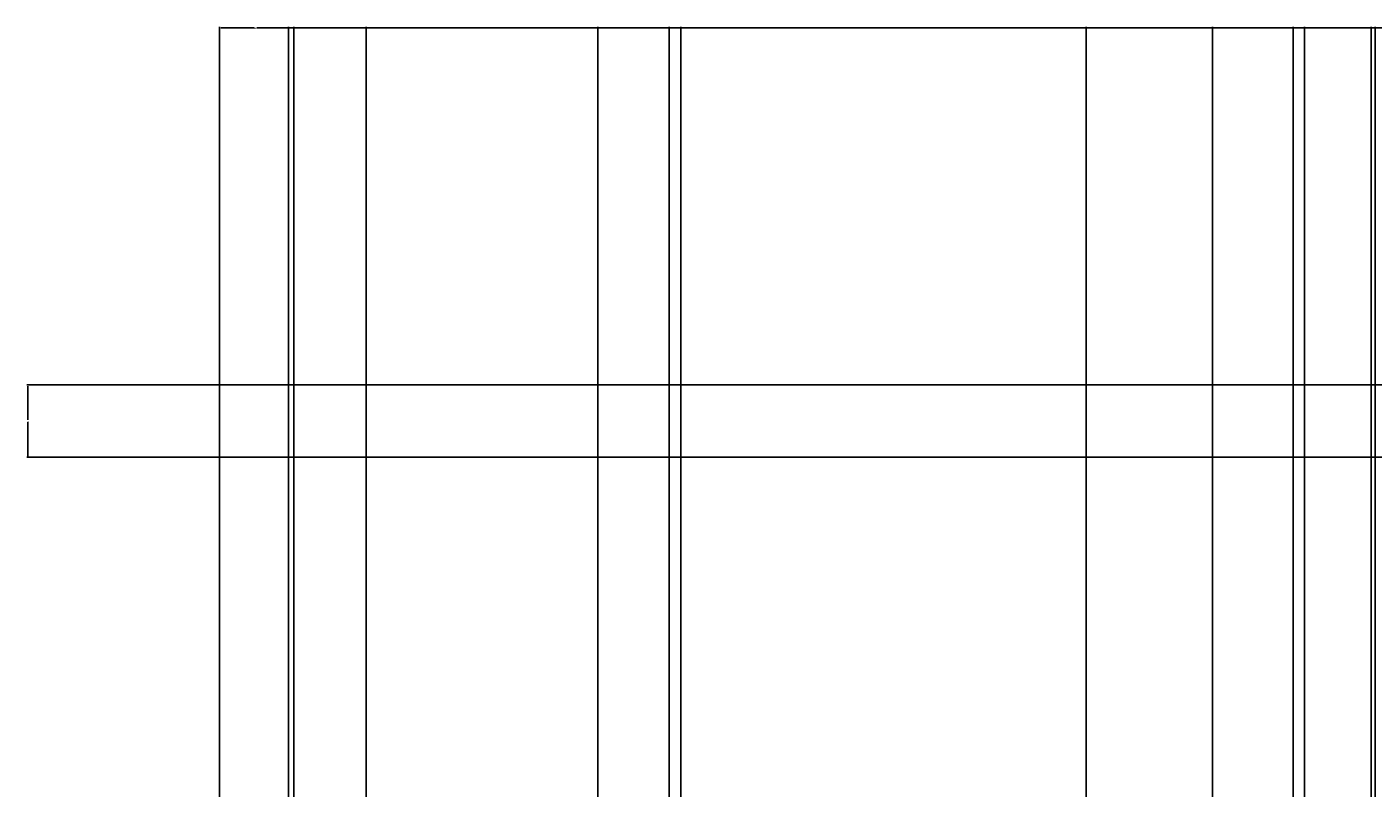
# Model space of a CAD drawing. Units: inches. Extents: x -8 to 554, y -200 to 499.
# Tile 8 of 12: x -8 to 216, y 372 to 499. Entities that reach past the tile are written whole.
import ezdxf

# ---------------------------------------------------------------- set-up
doc = ezdxf.new("R2010")
doc.units = ezdxf.units.IN
doc.header["$MEASUREMENT"] = 0
doc.layers.add('A-ANNO-DIMS', color=2, linetype='Continuous', lineweight=18)
doc.styles.get("Standard").update_dxf_attribs({"font": 'arial.ttf'})
doc.dimstyles.get("Standard").update_dxf_attribs({"dimtxt": 0.18, "dimasz": 0.18, "dimexe": 0.18, "dimexo": 0.0625, "dimgap": 0.09, "dimtad": 0, "dimtih": 1, "dimtoh": 1, "dimdec": 4, "dimzin": 0, "dimdsep": 46, "dimtxsty": 'Standard', "dimcen": 0.09, "dimadec": 0, "dimazin": 0, "dimtfac": 1, "dimtdec": 4, "dimtofl": 0, "dimtmove": 0, "dimatfit": 3, "dimfxl": 1, "dimtolj": 1, "dimtzin": 0, "dimarcsym": 0})

# ---------------------------------------------------------------- blocks, each defined once
blk = doc.blocks.new('*D40')
at = {"layer": 'A-ANNO-DIMS', "color": 0, "lineweight": -2, "transparency": 16777216}
for p, q in [((222.95, 439.48), (-7.69, 439.48)), ((-7.51, 439.3), (-7.51, 433.66)), ((-7.51, 427.66), (-7.51, 433.3)), ((222.95, 427.48), (-7.69, 427.48))]:
    blk.add_line(p, q, dxfattribs=at)
at = {"layer": 'A-ANNO-DIMS', "color": 0, "transparency": 16777216}
for points in [[(-7.54, 439.3), (-7.48, 439.3), (-7.51, 439.48)], [(-7.54, 427.66), (-7.48, 427.66), (-7.51, 427.48)]]:
    blk.add_solid(points, dxfattribs=at)
at = {"layer": 'Defpoints', "color": 0, "transparency": 16777216}
for p in [(223.01, 439.48), (-7.51, 427.48), (223.01, 427.48)]:
    blk.add_point(p, dxfattribs=at)
at = {"layer": 'A-ANNO-DIMS', "color": 0, "transparency": 16777216, "insert": (-7.51, 433.48), "char_height": 0.18, "attachment_point": 5}
blk.add_mtext('\\A1;12', dxfattribs=at)
blk = doc.blocks.new('*D42')
at = {"layer": 'A-ANNO-DIMS', "color": 0, "lineweight": -2, "transparency": 16777216}
for p, q in [((100.98, 319.33), (100.98, 498.99)), ((168.34, 319.54), (168.34, 498.99)), ((101.16, 498.81), (134.27, 498.81)), ((168.16, 498.81), (135.05, 498.81))]:
    blk.add_line(p, q, dxfattribs=at)
at = {"layer": 'A-ANNO-DIMS', "color": 0, "transparency": 16777216}
for points in [[(101.16, 498.84), (101.16, 498.78), (100.98, 498.81)], [(168.16, 498.84), (168.16, 498.78), (168.34, 498.81)]]:
    blk.add_solid(points, dxfattribs=at)
at = {"layer": 'Defpoints', "color": 0, "transparency": 16777216}
for p in [(168.34, 498.81), (100.98, 319.27), (168.34, 319.48)]:
    blk.add_point(p, dxfattribs=at)
at = {"layer": 'A-ANNO-DIMS', "color": 0, "transparency": 16777216, "insert": (134.66, 498.81), "char_height": 0.18, "attachment_point": 5}
blk.add_mtext('\\A1;67.37', dxfattribs=at)
blk = doc.blocks.new('*D43')
at = {"layer": 'A-ANNO-DIMS', "color": 0, "lineweight": -2, "transparency": 16777216}
for p, q in [((168.34, 319.54), (168.34, 498.99)), ((216.34, 319.54), (216.34, 498.99)), ((168.52, 498.81), (192.12, 498.81)), ((216.16, 498.81), (192.56, 498.81))]:
    blk.add_line(p, q, dxfattribs=at)
at = {"layer": 'A-ANNO-DIMS', "color": 0, "transparency": 16777216}
for points in [[(168.52, 498.84), (168.52, 498.78), (168.34, 498.81)], [(216.16, 498.84), (216.16, 498.78), (216.34, 498.81)]]:
    blk.add_solid(points, dxfattribs=at)
at = {"layer": 'Defpoints', "color": 0, "transparency": 16777216}
for p in [(216.34, 498.81), (168.34, 319.48), (216.34, 319.48)]:
    blk.add_point(p, dxfattribs=at)
at = {"layer": 'A-ANNO-DIMS', "color": 0, "transparency": 16777216, "insert": (192.34, 498.81), "char_height": 0.18, "attachment_point": 5}
blk.add_mtext('\\A1;48', dxfattribs=at)
blk = doc.blocks.new('*D55')
at = {"layer": 'A-ANNO-DIMS', "color": 0, "lineweight": -2, "transparency": 16777216}
for p, q in [((204.61, -30.61), (204.61, 498.99)), ((453.32, -30.61), (453.32, 498.99)), ((204.79, 498.81), (328.57, 498.81)), ((453.14, 498.81), (329.36, 498.81))]:
    blk.add_line(p, q, dxfattribs=at)
at = {"layer": 'A-ANNO-DIMS', "color": 0, "transparency": 16777216}
for points in [[(204.79, 498.84), (204.79, 498.78), (204.61, 498.81)], [(453.14, 498.84), (453.14, 498.78), (453.32, 498.81)]]:
    blk.add_solid(points, dxfattribs=at)
at = {"layer": 'Defpoints', "color": 0, "transparency": 16777216}
for p in [(453.32, 498.81), (204.61, -30.67), (453.32, -30.67)]:
    blk.add_point(p, dxfattribs=at)
at = {"layer": 'A-ANNO-DIMS', "color": 0, "transparency": 16777216, "insert": (328.96, 498.81), "char_height": 0.18, "attachment_point": 5}
blk.add_mtext('\\A1;248.7', dxfattribs=at)
blk = doc.blocks.new('*D56')
at = {"layer": 'A-ANNO-DIMS', "color": 0, "lineweight": -2, "transparency": 16777216}
for p, q in [((24.34, 7.54), (24.34, 498.99)), ((36.69, 7.54), (36.69, 498.99)), ((24.52, 498.81), (30.06, 498.81)), ((36.51, 498.81), (30.97, 498.81))]:
    blk.add_line(p, q, dxfattribs=at)
at = {"layer": 'A-ANNO-DIMS', "color": 0, "transparency": 16777216}
for points in [[(24.52, 498.84), (24.52, 498.78), (24.34, 498.81)], [(36.51, 498.84), (36.51, 498.78), (36.69, 498.81)]]:
    blk.add_solid(points, dxfattribs=at)
at = {"layer": 'Defpoints', "color": 0, "transparency": 16777216}
for p in [(36.69, 498.81), (24.34, 7.48), (36.69, 7.48)]:
    blk.add_point(p, dxfattribs=at)
at = {"layer": 'A-ANNO-DIMS', "color": 0, "transparency": 16777216, "insert": (30.52, 498.81), "char_height": 0.18, "attachment_point": 5}
blk.add_mtext('\\A1;12.346', dxfattribs=at)
blk = doc.blocks.new('*D57')
at = {"layer": 'A-ANNO-DIMS', "color": 0, "lineweight": -2, "transparency": 16777216}
for p, q in [((36.69, -52.46), (36.69, 498.99)), ((48.69, -52.46), (48.69, 498.99)), ((36.87, 498.81), (42.48, 498.81)), ((48.51, 498.81), (42.9, 498.81))]:
    blk.add_line(p, q, dxfattribs=at)
at = {"layer": 'A-ANNO-DIMS', "color": 0, "transparency": 16777216}
for points in [[(36.87, 498.84), (36.87, 498.78), (36.69, 498.81)], [(48.51, 498.84), (48.51, 498.78), (48.69, 498.81)]]:
    blk.add_solid(points, dxfattribs=at)
at = {"layer": 'Defpoints', "color": 0, "transparency": 16777216}
for p in [(48.69, 498.81), (36.69, -52.52), (48.69, -52.52)]:
    blk.add_point(p, dxfattribs=at)
at = {"layer": 'A-ANNO-DIMS', "color": 0, "transparency": 16777216, "insert": (42.69, 498.81), "char_height": 0.18, "attachment_point": 5}
blk.add_mtext('\\A1;12', dxfattribs=at)
blk = doc.blocks.new('*D58')
at = {"layer": 'A-ANNO-DIMS', "color": 0, "lineweight": -2, "transparency": 16777216}
for p, q in [((36.69, 7.54), (36.69, 498.99)), ((87.21, 7.54), (87.21, 498.99)), ((36.87, 498.81), (61.56, 498.81)), ((87.03, 498.81), (62.34, 498.81))]:
    blk.add_line(p, q, dxfattribs=at)
at = {"layer": 'A-ANNO-DIMS', "color": 0, "transparency": 16777216}
for points in [[(36.87, 498.84), (36.87, 498.78), (36.69, 498.81)], [(87.03, 498.84), (87.03, 498.78), (87.21, 498.81)]]:
    blk.add_solid(points, dxfattribs=at)
at = {"layer": 'Defpoints', "color": 0, "transparency": 16777216}
for p in [(87.21, 498.81), (36.69, 7.48), (87.21, 7.48)]:
    blk.add_point(p, dxfattribs=at)
at = {"layer": 'A-ANNO-DIMS', "color": 0, "transparency": 16777216, "insert": (61.95, 498.81), "char_height": 0.18, "attachment_point": 5}
blk.add_mtext('\\A1;50.52', dxfattribs=at)
blk = doc.blocks.new('*D59')
at = {"layer": 'A-ANNO-DIMS', "color": 0, "lineweight": -2, "transparency": 16777216}
for p, q in [((87.21, -60.84), (87.21, 498.99)), ((99.04, -60.84), (99.04, 498.99)), ((87.39, 498.81), (92.67, 498.81)), ((98.86, 498.81), (93.58, 498.81))]:
    blk.add_line(p, q, dxfattribs=at)
at = {"layer": 'A-ANNO-DIMS', "color": 0, "transparency": 16777216}
for points in [[(87.39, 498.84), (87.39, 498.78), (87.21, 498.81)], [(98.86, 498.84), (98.86, 498.78), (99.04, 498.81)]]:
    blk.add_solid(points, dxfattribs=at)
at = {"layer": 'Defpoints', "color": 0, "transparency": 16777216}
for p in [(99.04, 498.81), (87.21, -60.9), (99.04, -60.9)]:
    blk.add_point(p, dxfattribs=at)
at = {"layer": 'A-ANNO-DIMS', "color": 0, "transparency": 16777216, "insert": (93.12, 498.81), "char_height": 0.18, "attachment_point": 5}
blk.add_mtext('\\A1;11.827', dxfattribs=at)
blk = doc.blocks.new('*D60')
at = {"layer": 'A-ANNO-DIMS', "color": 0, "lineweight": -2, "transparency": 16777216}
for p, q in [((87.21, 7.54), (87.21, 498.99)), ((189.3, 7.54), (189.3, 498.99)), ((87.39, 498.81), (137.89, 498.81)), ((189.12, 498.81), (138.63, 498.81))]:
    blk.add_line(p, q, dxfattribs=at)
at = {"layer": 'A-ANNO-DIMS', "color": 0, "transparency": 16777216}
for points in [[(87.39, 498.84), (87.39, 498.78), (87.21, 498.81)], [(189.12, 498.84), (189.12, 498.78), (189.3, 498.81)]]:
    blk.add_solid(points, dxfattribs=at)
at = {"layer": 'Defpoints', "color": 0, "transparency": 16777216}
for p in [(189.3, 498.81), (87.21, 7.48), (189.3, 7.48)]:
    blk.add_point(p, dxfattribs=at)
at = {"layer": 'A-ANNO-DIMS', "color": 0, "transparency": 16777216, "insert": (138.26, 498.81), "char_height": 0.18, "attachment_point": 5}
blk.add_mtext('\\A1;102.1', dxfattribs=at)
blk = doc.blocks.new('*D61')
at = {"layer": 'A-ANNO-DIMS', "color": 0, "lineweight": -2, "transparency": 16777216}
for p, q in [((189.3, -52.46), (189.3, 498.99)), ((202.75, -52.46), (202.75, 498.99)), ((189.48, 498.81), (195.57, 498.81)), ((202.57, 498.81), (196.48, 498.81))]:
    blk.add_line(p, q, dxfattribs=at)
at = {"layer": 'A-ANNO-DIMS', "color": 0, "transparency": 16777216}
for points in [[(189.48, 498.84), (189.48, 498.78), (189.3, 498.81)], [(202.57, 498.84), (202.57, 498.78), (202.75, 498.81)]]:
    blk.add_solid(points, dxfattribs=at)
at = {"layer": 'Defpoints', "color": 0, "transparency": 16777216}
for p in [(202.75, 498.81), (189.3, -52.52), (202.75, -52.52)]:
    blk.add_point(p, dxfattribs=at)
at = {"layer": 'A-ANNO-DIMS', "color": 0, "transparency": 16777216, "insert": (196.03, 498.81), "char_height": 0.18, "attachment_point": 5}
blk.add_mtext('\\A1;13.446', dxfattribs=at)
blk = doc.blocks.new('*D62')
at = {"layer": 'A-ANNO-DIMS', "color": 0, "lineweight": -2, "transparency": 16777216}
for p, q in [((189.3, 7.54), (189.3, 498.99)), ((337.49, 7.54), (337.49, 498.99)), ((189.48, 498.81), (263.01, 498.81)), ((337.31, 498.81), (263.78, 498.81))]:
    blk.add_line(p, q, dxfattribs=at)
at = {"layer": 'A-ANNO-DIMS', "color": 0, "transparency": 16777216}
for points in [[(189.48, 498.84), (189.48, 498.78), (189.3, 498.81)], [(337.31, 498.84), (337.31, 498.78), (337.49, 498.81)]]:
    blk.add_solid(points, dxfattribs=at)
at = {"layer": 'Defpoints', "color": 0, "transparency": 16777216}
for p in [(337.49, 498.81), (189.3, 7.48), (337.49, 7.48)]:
    blk.add_point(p, dxfattribs=at)
at = {"layer": 'A-ANNO-DIMS', "color": 0, "transparency": 16777216, "insert": (263.4, 498.81), "char_height": 0.18, "attachment_point": 5}
blk.add_mtext('\\A1;148.2', dxfattribs=at)
blk = doc.blocks.new('*D70')
at = {"layer": 'A-ANNO-DIMS', "color": 0, "lineweight": -2, "transparency": 16777216}
for p, q in [((35.79, 357.7), (35.79, 498.99)), ((215.68, 357.7), (215.68, 498.99)), ((35.97, 498.81), (125.35, 498.81)), ((215.5, 498.81), (126.12, 498.81))]:
    blk.add_line(p, q, dxfattribs=at)
at = {"layer": 'A-ANNO-DIMS', "color": 0, "transparency": 16777216}
for points in [[(35.97, 498.84), (35.97, 498.78), (35.79, 498.81)], [(215.5, 498.84), (215.5, 498.78), (215.68, 498.81)]]:
    blk.add_solid(points, dxfattribs=at)
at = {"layer": 'Defpoints', "color": 0, "transparency": 16777216}
for p in [(215.68, 498.81), (35.79, 357.64), (215.68, 357.64)]:
    blk.add_point(p, dxfattribs=at)
at = {"layer": 'A-ANNO-DIMS', "color": 0, "transparency": 16777216, "insert": (125.73, 498.81), "char_height": 0.18, "attachment_point": 5}
blk.add_mtext('\\A1;179.9', dxfattribs=at)
blk = doc.blocks.new('*D72')
at = {"layer": 'A-ANNO-DIMS', "color": 0, "lineweight": -2, "transparency": 16777216}
for p, q in [((24.34, 371.85), (24.34, 498.99)), ((35.79, 371.85), (35.79, 498.99)), ((24.52, 498.81), (29.61, 498.81)), ((35.61, 498.81), (30.52, 498.81))]:
    blk.add_line(p, q, dxfattribs=at)
at = {"layer": 'A-ANNO-DIMS', "color": 0, "transparency": 16777216}
for points in [[(24.52, 498.84), (24.52, 498.78), (24.34, 498.81)], [(35.61, 498.84), (35.61, 498.78), (35.79, 498.81)]]:
    blk.add_solid(points, dxfattribs=at)
at = {"layer": 'Defpoints', "color": 0, "transparency": 16777216}
for p in [(35.79, 498.81), (24.34, 371.79), (35.79, 371.79)]:
    blk.add_point(p, dxfattribs=at)
at = {"layer": 'A-ANNO-DIMS', "color": 0, "transparency": 16777216, "insert": (30.06, 498.81), "char_height": 0.18, "attachment_point": 5}
blk.add_mtext('\\A1;11.445', dxfattribs=at)

msp = doc.modelspace()

# ---------------------------------------------------------------- dimensions: what is measured, and where the dimension line sits
at = {"layer": 'A-ANNO-DIMS'}
for base, p1, p2, override, picture, middle in [((36.6882, 498.8091), (24.3421, 7.4814), (36.6882, 7.4814), {"dimdec": 3, "dimlfac": 1, "dimrnd": 0, "dimzin": 0, "dimdsep": 46, "dimlunit": 2}, '*D56', (30.5151, 498.8091)), ((35.7874, 498.8091), (24.3421, 371.7921), (35.7874, 371.7921), {"dimdec": 3, "dimlfac": 1, "dimrnd": 0, "dimzin": 0, "dimdsep": 46, "dimlunit": 2}, '*D72', (30.0647, 498.8091)), ((215.6778, 498.8091), (35.7874, 357.6367), (215.6778, 357.6367), {"dimdec": 1, "dimlfac": 1, "dimrnd": 0, "dimzin": 0, "dimdsep": 46, "dimlunit": 2}, '*D70', (125.7326, 498.8091)), ((48.6882, 498.8091), (36.6882, -52.5186), (48.6882, -52.5186), {"dimdec": 0, "dimlfac": 1, "dimrnd": 0, "dimzin": 0, "dimdsep": 46, "dimlunit": 2}, '*D57', (42.6882, 498.8091)), ((87.21, 498.8091), (36.6882, 7.4814), (87.21, 7.4814), {"dimdec": 2, "dimlfac": 1, "dimrnd": 0, "dimzin": 0, "dimdsep": 46, "dimlunit": 2}, '*D58', (61.9491, 498.8091)), ((99.037, 498.8091), (87.21, -60.9032), (99.037, -60.9032), {"dimdec": 3, "dimlfac": 1, "dimrnd": 0, "dimzin": 0, "dimdsep": 46, "dimlunit": 2}, '*D59', (93.1235, 498.8091)), ((189.3049, 498.8091), (87.21, 7.4814), (189.3049, 7.4814), {"dimdec": 1, "dimlfac": 1, "dimrnd": 0, "dimzin": 0, "dimdsep": 46, "dimlunit": 2}, '*D60', (138.2575, 498.8091)), ((168.3421, 498.8091), (100.9765, 319.2713), (168.3421, 319.4814), {"dimdec": 2, "dimlfac": 1, "dimrnd": 0, "dimzin": 0, "dimdsep": 46, "dimlunit": 2}, '*D42', (134.6593, 498.8091)), ((216.3421, 498.8091), (168.3421, 319.4814), (216.3421, 319.4814), {"dimdec": 0, "dimlfac": 1, "dimrnd": 0, "dimzin": 0, "dimdsep": 46, "dimlunit": 2}, '*D43', (192.3421, 498.8091)), ((202.7513, 498.8091), (189.3049, -52.5186), (202.7513, -52.5186), {"dimdec": 3, "dimlfac": 1, "dimrnd": 0, "dimzin": 0, "dimdsep": 46, "dimlunit": 2}, '*D61', (196.0281, 498.8091)), ((337.4923, 498.8091), (189.3049, 7.4814), (337.4923, 7.4814), {"dimdec": 1, "dimlfac": 1, "dimrnd": 0, "dimzin": 0, "dimdsep": 46, "dimlunit": 2}, '*D62', (263.3986, 498.8091)), ((453.3222, 498.8091), (204.6055, -30.6677), (453.3222, -30.6677), {"dimdec": 1, "dimlfac": 1, "dimrnd": 0, "dimzin": 0, "dimdsep": 46, "dimlunit": 2}, '*D55', (328.9639, 498.8091))]:
    dim = msp.add_linear_dim(base=base, p1=p1, p2=p2, dimstyle='Standard', override=override, dxfattribs=at)
    dim.commit()
    dim.dimension.update_dxf_attribs({"geometry": picture, "text_midpoint": middle})
dim = msp.add_linear_dim(base=(-7.5079, 427.4814), p1=(223.0104, 439.4814), p2=(223.0104, 427.4814), angle=90, dimstyle='Standard', override={"dimdec": 0, "dimlfac": 1, "dimrnd": 0, "dimzin": 0, "dimdsep": 46, "dimlunit": 2}, dxfattribs=at)
dim.commit()
dim.dimension.update_dxf_attribs({"geometry": '*D40', "text_midpoint": (-7.5079, 433.4814)})

doc.saveas('drawing.dxf')
